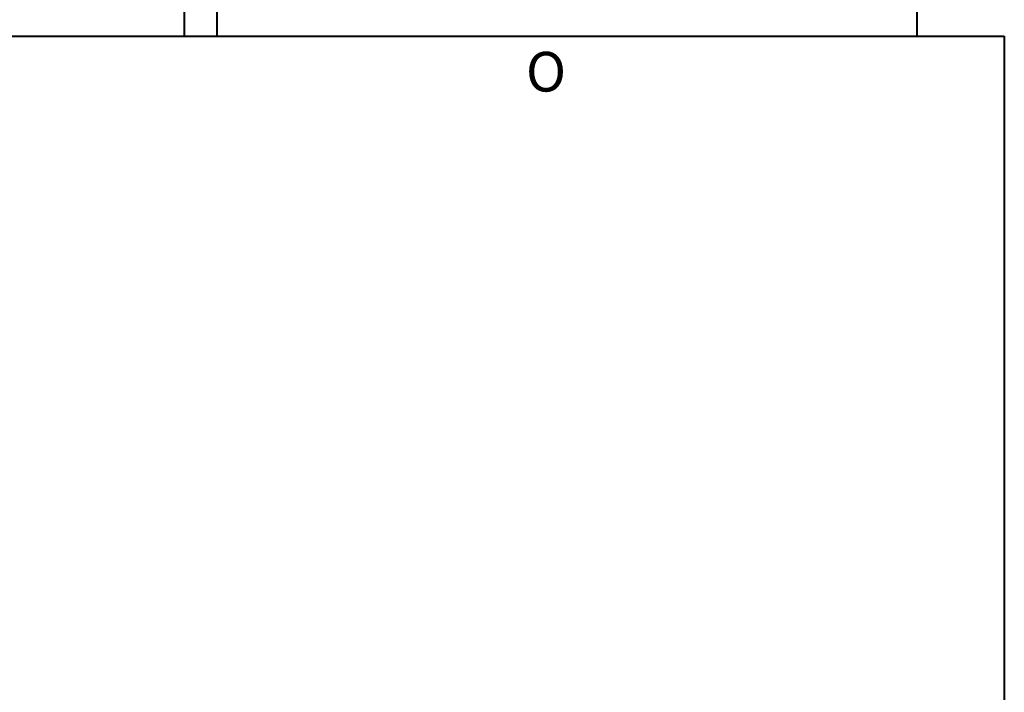
# Model space of a CAD drawing. Units: inches. Extents: x 182 to 1022, y -617 to 111.
# Tile 16 of 33: x 294 to 429, y -212 to -120. Entities that reach past the tile are written whole.
import ezdxf

# ---------------------------------------------------------------- set-up
doc = ezdxf.new("R2010")
doc.units = ezdxf.units.IN
doc.header["$MEASUREMENT"] = 0
doc.layers.add('A-ANNO-IDEN', color=1, linetype='Continuous', lineweight=18)
doc.layers.add('wall', color=1, linetype='Continuous', lineweight=40)
doc.styles.get("Standard").update_dxf_attribs({"font": 'arial.ttf'})

msp = doc.modelspace()

# ---------------------------------------------------------------- linework, layer by layer
at = {"layer": 'wall'}
for p, q in [((316.36, -9.37), (316.36, -121.87)), ((320.86, -9.37), (320.86, -121.87)), ((416.86, -117.37), (416.86, -121.87)), ((238.36, -121.87), (428.86, -121.87)), ((428.86, -121.87), (428.86, -246.37))]:
    msp.add_line(p, q, dxfattribs=at)

# ---------------------------------------------------------------- texts
at = {"layer": 'A-ANNO-IDEN'}
msp.add_text('O', height=5.44, dxfattribs=at).set_placement((363.26, -129.48))

doc.saveas('drawing.dxf')
